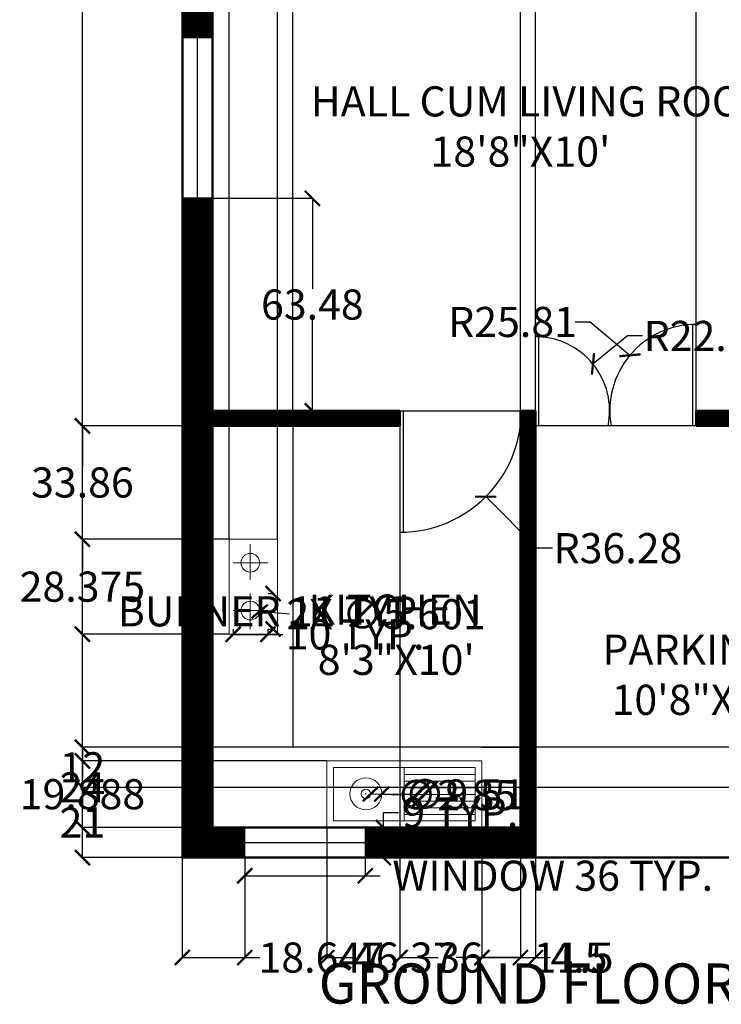
# Model space of a CAD drawing. Units: inches. Extents: x 104 to 466, y -74 to 547.
# Tile 1 of 4: x 110 to 320, y -74 to 220. Entities that reach past the tile are written whole.
import ezdxf

# ---------------------------------------------------------------- set-up
doc = ezdxf.new("R2010")
doc.units = ezdxf.units.IN
doc.header["$MEASUREMENT"] = 0
for name, color, linetype, lineweight in [('A-ANNO-DIMS', 2, 'Continuous', 18), ('A-ANNO-TEXT', 7, 'Continuous', 35), ('A-AREA-IDEN', 7, 'Continuous', 25), ('A-DOOR', 3, 'Continuous', 25), ('A-EQPM', 9, 'Continuous', 18), ('A-FLOR-CASE', 8, 'Continuous', 25), ('A-FLOR-FIXT', 8, 'Continuous', 18), ('A-GLAZ', 4, 'Continuous', 25), ('A-WALL', 7, 'Continuous', 50), ('A-WALL-PATT', 8, 'Continuous', 13)]:
    doc.layers.add(name, color=color, linetype=linetype, lineweight=lineweight)
doc.styles.get("Standard").update_dxf_attribs({"font": 'arial.ttf'})
doc.dimstyles.get("Standard").update_dxf_attribs({"dimtxt": 9, "dimasz": 4.5, "dimexe": 0.18, "dimexo": 0.0625, "dimgap": 0.09, "dimtad": 0, "dimtih": 1, "dimtoh": 1, "dimdec": 1, "dimzin": 0, "dimdsep": 46, "dimlunit": 4, "dimtxsty": 'Standard', "dimblk": 'ARCHTICK', "dimcen": 0.09, "dimadec": 0, "dimazin": 0, "dimtfac": 1, "dimtdec": 1, "dimtofl": 0, "dimtmove": 0, "dimatfit": 3, "dimfxl": 1, "dimtolj": 1, "dimtzin": 0, "dimarcsym": 0})

# ---------------------------------------------------------------- blocks, each defined once
blk = doc.blocks.new('WINDOW-48IN')
for p, q in [((0, 48), (9, 48)), ((0, 0), (0, 48)), ((4.5, 48), (4.5, 0)), ((9, 48), (9, 0)), ((9, 0), (0, 0))]:
    blk.add_line(p, q)
blk = doc.blocks.new('WINDOW-36IN')
for p, q in [((0, 9), (36, 9)), ((0, 0), (0, 9)), ((36, 9), (36, 0)), ((0, 4.5), (36, 4.5)), ((36, 0), (0, 0))]:
    blk.add_line(p, q)
blk = doc.blocks.new('COOKTOP-BURNER')
for q in [(5.16, 10.61), (0, 5.52), (5.16, 0), (10.39, 5.52)]:
    blk.add_line((5.16, 5.52), q)
blk.add_circle((5.16, 5.52), 2.8)
blk = doc.blocks.new('_ArchTick')
at = {"color": 0, "linetype": 'ByBlock', "const_width": 0.15}
blk.add_lwpolyline([(-0.5, -0.5), (0.5, 0.5)], dxfattribs=at)
blk = doc.blocks.new('*D9')
at = {"layer": 'A-ANNO-DIMS', "color": 0, "lineweight": -2, "transparency": 16777216}
for p, q in [((177.73, -30.52), (177.73, -36.04)), ((213.73, -30.52), (213.73, -36.04)), ((177.73, -35.86), (213.73, -35.86)), ((213.73, -35.86), (218.23, -35.86))]:
    blk.add_line(p, q, dxfattribs=at)
at = {"layer": 'Defpoints', "color": 0, "transparency": 16777216}
for p in [(177.73, -30.46), (213.73, -30.46), (213.73, -35.86)]:
    blk.add_point(p, dxfattribs=at)
at = {"layer": 'A-ANNO-DIMS', "color": 0, "lineweight": -2, "transparency": 16777216, "xscale": 4.5, "yscale": 4.5, "zscale": 4.5, "rotation": 180}
blk.add_blockref('_ArchTick', (177.73, -35.86), dxfattribs=at)
at = {"layer": 'A-ANNO-DIMS', "color": 0, "lineweight": -2, "transparency": 16777216, "xscale": 4.5, "yscale": 4.5, "zscale": 4.5}
blk.add_blockref('_ArchTick', (213.73, -35.86), dxfattribs=at)
at = {"layer": 'A-ANNO-DIMS', "color": 0, "transparency": 16777216, "insert": (269.74, -35.86), "char_height": 9, "attachment_point": 5}
blk.add_mtext('\\A1;WINDOW 36 TYP.', dxfattribs=at)
blk = doc.blocks.new('*D10')
at = {"layer": 'A-ANNO-DIMS', "color": 0, "lineweight": -2, "transparency": 16777216}
for p, q in [((219.13, -21.46), (219.13, -16.96)), ((219.13, -16.96), (223.63, -16.96)), ((213.79, -21.46), (219.31, -21.46)), ((219.13, -30.46), (219.13, -21.46)), ((213.79, -30.46), (219.31, -30.46))]:
    blk.add_line(p, q, dxfattribs=at)
at = {"layer": 'Defpoints', "color": 0, "transparency": 16777216}
for p in [(213.73, -21.46), (219.13, -21.46), (213.73, -30.46)]:
    blk.add_point(p, dxfattribs=at)
at = {"layer": 'A-ANNO-DIMS', "color": 0, "lineweight": -2, "transparency": 16777216, "xscale": 4.5, "yscale": 4.5, "zscale": 4.5}
for p, rotation in [((219.13, -21.46), 90), ((219.13, -30.46), 270)]:
    blk.add_blockref('_ArchTick', p, dxfattribs=dict(at, rotation=rotation))
at = {"layer": 'A-ANNO-DIMS', "color": 0, "transparency": 16777216, "insert": (242.13, -16.96), "char_height": 9, "attachment_point": 5}
blk.add_mtext('\\A1;9 TYP.', dxfattribs=at)
blk = doc.blocks.new('*D15')
at = {"layer": 'A-ANNO-DIMS', "color": 0, "lineweight": -2, "transparency": 16777216}
for p, q in [((184.68, 48.44), (186.39, 48.44)), ((186.21, 48.44), (186.21, 47.82)), ((186.21, 37.84), (186.21, 38.45)), ((184.68, 37.84), (186.39, 37.84))]:
    blk.add_line(p, q, dxfattribs=at)
at = {"layer": 'Defpoints', "color": 0, "transparency": 16777216}
for p in [(184.62, 48.44), (186.21, 48.44), (184.62, 37.84)]:
    blk.add_point(p, dxfattribs=at)
at = {"layer": 'A-ANNO-DIMS', "color": 0, "lineweight": -2, "transparency": 16777216, "xscale": 4.5, "yscale": 4.5, "zscale": 4.5}
for p, rotation in [((186.21, 48.44), 90), ((186.21, 37.84), 270)]:
    blk.add_blockref('_ArchTick', p, dxfattribs=dict(at, rotation=rotation))
at = {"layer": 'A-ANNO-DIMS', "color": 0, "transparency": 16777216, "insert": (186.21, 43.14), "char_height": 9, "attachment_point": 5}
blk.add_mtext('\\A1;BURNER 11 TYP.', dxfattribs=at)
blk = doc.blocks.new('*D16')
at = {"layer": 'A-ANNO-DIMS', "color": 0, "lineweight": -2, "transparency": 16777216}
for p, q in [((174.23, 37.77), (174.23, 36.06)), ((174.23, 36.24), (184.62, 36.24)), ((184.62, 37.77), (184.62, 36.06)), ((184.62, 36.24), (189.12, 36.24))]:
    blk.add_line(p, q, dxfattribs=at)
at = {"layer": 'Defpoints', "color": 0, "transparency": 16777216}
for p in [(174.23, 37.84), (184.62, 37.84), (184.62, 36.24)]:
    blk.add_point(p, dxfattribs=at)
at = {"layer": 'A-ANNO-DIMS', "color": 0, "lineweight": -2, "transparency": 16777216, "xscale": 4.5, "yscale": 4.5, "zscale": 4.5, "rotation": 180}
blk.add_blockref('_ArchTick', (174.23, 36.24), dxfattribs=at)
at = {"layer": 'A-ANNO-DIMS', "color": 0, "lineweight": -2, "transparency": 16777216, "xscale": 4.5, "yscale": 4.5, "zscale": 4.5}
blk.add_blockref('_ArchTick', (184.62, 36.24), dxfattribs=at)
at = {"layer": 'A-ANNO-DIMS', "color": 0, "transparency": 16777216, "insert": (210.69, 36.24), "char_height": 9, "attachment_point": 5}
blk.add_mtext('\\A1;10 TYP.', dxfattribs=at)
blk = doc.blocks.new('*D18')
at = {"layer": 'A-ANNO-DIMS', "color": 0, "lineweight": -2, "transparency": 16777216}
for p, q in [((159.02, 511.04), (129.05, 511.04)), ((129.23, 511.04), (129.23, 244.98)), ((129.23, -30.46), (129.23, 235.61)), ((159.02, -30.46), (129.05, -30.46))]:
    blk.add_line(p, q, dxfattribs=at)
at = {"layer": 'Defpoints', "color": 0, "transparency": 16777216}
for p in [(129.23, 511.04), (159.08, 511.04), (159.08, -30.46)]:
    blk.add_point(p, dxfattribs=at)
at = {"layer": 'A-ANNO-DIMS', "color": 0, "lineweight": -2, "transparency": 16777216, "xscale": 4.5, "yscale": 4.5, "zscale": 4.5}
for p, rotation in [((129.23, 511.04), 90), ((129.23, -30.46), 270)]:
    blk.add_blockref('_ArchTick', p, dxfattribs=dict(at, rotation=rotation))
at = {"layer": 'A-ANNO-DIMS', "color": 0, "transparency": 16777216, "insert": (129.23, 240.29), "char_height": 9, "attachment_point": 5}
blk.add_mtext('\\A1;541.5', dxfattribs=at)
blk = doc.blocks.new('*D19')
at = {"layer": 'A-ANNO-DIMS', "color": 0, "lineweight": -2, "transparency": 16777216}
for p, q in [((159.08, -30.52), (159.08, -60.49)), ((177.73, -30.52), (177.73, -60.49)), ((159.08, -60.31), (177.73, -60.31)), ((177.73, -60.31), (182.23, -60.31))]:
    blk.add_line(p, q, dxfattribs=at)
at = {"layer": 'Defpoints', "color": 0, "transparency": 16777216}
for p in [(159.08, -30.46), (177.73, -30.46), (177.73, -60.31)]:
    blk.add_point(p, dxfattribs=at)
at = {"layer": 'A-ANNO-DIMS', "color": 0, "lineweight": -2, "transparency": 16777216, "xscale": 4.5, "yscale": 4.5, "zscale": 4.5, "rotation": 180}
blk.add_blockref('_ArchTick', (159.08, -60.31), dxfattribs=at)
at = {"layer": 'A-ANNO-DIMS', "color": 0, "lineweight": -2, "transparency": 16777216, "xscale": 4.5, "yscale": 4.5, "zscale": 4.5}
blk.add_blockref('_ArchTick', (177.73, -60.31), dxfattribs=at)
at = {"layer": 'A-ANNO-DIMS', "color": 0, "transparency": 16777216, "insert": (200.58, -60.31), "char_height": 9, "attachment_point": 5}
blk.add_mtext('\\A1;18.647', dxfattribs=at)
blk = doc.blocks.new('*D21')
at = {"layer": 'A-ANNO-DIMS', "color": 0, "lineweight": -2, "transparency": 16777216}
for p, q in [((168.15, 166.52), (198.11, 166.52)), ((197.93, 166.52), (197.93, 139.47)), ((197.93, 103.04), (197.93, 130.1)), ((168.15, 103.04), (198.11, 103.04))]:
    blk.add_line(p, q, dxfattribs=at)
at = {"layer": 'Defpoints', "color": 0, "transparency": 16777216}
for p in [(168.08, 166.52), (168.08, 103.04), (197.93, 103.04)]:
    blk.add_point(p, dxfattribs=at)
at = {"layer": 'A-ANNO-DIMS', "color": 0, "lineweight": -2, "transparency": 16777216, "xscale": 4.5, "yscale": 4.5, "zscale": 4.5}
for p, rotation in [((197.93, 166.52), 90), ((197.93, 103.04), 270)]:
    blk.add_blockref('_ArchTick', p, dxfattribs=dict(at, rotation=rotation))
at = {"layer": 'A-ANNO-DIMS', "color": 0, "transparency": 16777216, "insert": (197.93, 134.78), "char_height": 9, "attachment_point": 5}
blk.add_mtext('\\A1;63.48', dxfattribs=at)
blk = doc.blocks.new('*D26')
at = {"layer": 'A-ANNO-DIMS', "color": 0, "lineweight": -2, "transparency": 16777216}
for p, q in [((168.08, 98.61), (168.08, 541.07)), ((168.08, 540.89), (207.59, 540.89)), ((260.08, 540.89), (220.57, 540.89)), ((260.08, 103.11), (260.08, 541.07))]:
    blk.add_line(p, q, dxfattribs=at)
at = {"layer": 'Defpoints', "color": 0, "transparency": 16777216}
for p in [(260.08, 540.89), (260.08, 103.04), (168.08, 98.54)]:
    blk.add_point(p, dxfattribs=at)
at = {"layer": 'A-ANNO-DIMS', "color": 0, "lineweight": -2, "transparency": 16777216, "xscale": 4.5, "yscale": 4.5, "zscale": 4.5, "rotation": 180}
blk.add_blockref('_ArchTick', (168.08, 540.89), dxfattribs=at)
at = {"layer": 'A-ANNO-DIMS', "color": 0, "lineweight": -2, "transparency": 16777216, "xscale": 4.5, "yscale": 4.5, "zscale": 4.5}
blk.add_blockref('_ArchTick', (260.08, 540.89), dxfattribs=at)
at = {"layer": 'A-ANNO-DIMS', "color": 0, "transparency": 16777216, "insert": (214.08, 540.89), "char_height": 9, "attachment_point": 5}
blk.add_mtext('\\A1;92', dxfattribs=at)
blk = doc.blocks.new('*D27')
at = {"layer": 'A-ANNO-DIMS', "color": 0, "lineweight": -2, "transparency": 16777216}
for p, q in [((260.08, -21.52), (260.08, -60.49)), ((264.58, -30.52), (264.58, -60.49)), ((260.08, -60.31), (264.58, -60.31)), ((264.58, -60.31), (269.08, -60.31))]:
    blk.add_line(p, q, dxfattribs=at)
at = {"layer": 'Defpoints', "color": 0, "transparency": 16777216}
for p in [(260.08, -21.46), (264.58, -30.46), (264.58, -60.31)]:
    blk.add_point(p, dxfattribs=at)
at = {"layer": 'A-ANNO-DIMS', "color": 0, "lineweight": -2, "transparency": 16777216, "xscale": 4.5, "yscale": 4.5, "zscale": 4.5, "rotation": 180}
blk.add_blockref('_ArchTick', (260.08, -60.31), dxfattribs=at)
at = {"layer": 'A-ANNO-DIMS', "color": 0, "lineweight": -2, "transparency": 16777216, "xscale": 4.5, "yscale": 4.5, "zscale": 4.5}
blk.add_blockref('_ArchTick', (264.58, -60.31), dxfattribs=at)
at = {"layer": 'A-ANNO-DIMS', "color": 0, "transparency": 16777216, "insert": (277.58, -60.31), "char_height": 9, "attachment_point": 5}
blk.add_mtext('\\A1;4.5', dxfattribs=at)
blk = doc.blocks.new('*D30')
at = {"layer": 'A-ANNO-DIMS', "color": 0, "lineweight": -2, "transparency": 16777216}
for p, q in [((368.52, 2.54), (129.05, 2.54)), ((129.23, 2.54), (129.23, 1.15)), ((129.23, -9.46), (129.23, -8.06)), ((368.52, -9.46), (129.05, -9.46))]:
    blk.add_line(p, q, dxfattribs=at)
at = {"layer": 'Defpoints', "color": 0, "transparency": 16777216}
for p in [(129.23, 2.54), (368.58, 2.54), (368.58, -9.46)]:
    blk.add_point(p, dxfattribs=at)
at = {"layer": 'A-ANNO-DIMS', "color": 0, "lineweight": -2, "transparency": 16777216, "xscale": 4.5, "yscale": 4.5, "zscale": 4.5}
for p, rotation in [((129.23, 2.54), 90), ((129.23, -9.46), 270)]:
    blk.add_blockref('_ArchTick', p, dxfattribs=dict(at, rotation=rotation))
at = {"layer": 'A-ANNO-DIMS', "color": 0, "transparency": 16777216, "insert": (129.23, -3.46), "char_height": 9, "attachment_point": 5}
blk.add_mtext('\\A1;12', dxfattribs=at)
blk = doc.blocks.new('*D31')
at = {"layer": 'A-ANNO-DIMS', "color": 0, "lineweight": -2, "transparency": 16777216}
for p, q in [((168.08, 98.61), (168.08, 541.07)), ((168.08, 540.89), (173.49, 540.89)), ((192.08, 540.89), (186.68, 540.89)), ((192.08, 98.61), (192.08, 541.07))]:
    blk.add_line(p, q, dxfattribs=at)
at = {"layer": 'Defpoints', "color": 0, "transparency": 16777216}
for p in [(192.08, 540.89), (168.08, 98.54), (192.08, 98.54)]:
    blk.add_point(p, dxfattribs=at)
at = {"layer": 'A-ANNO-DIMS', "color": 0, "lineweight": -2, "transparency": 16777216, "xscale": 4.5, "yscale": 4.5, "zscale": 4.5, "rotation": 180}
blk.add_blockref('_ArchTick', (168.08, 540.89), dxfattribs=at)
at = {"layer": 'A-ANNO-DIMS', "color": 0, "lineweight": -2, "transparency": 16777216, "xscale": 4.5, "yscale": 4.5, "zscale": 4.5}
blk.add_blockref('_ArchTick', (192.08, 540.89), dxfattribs=at)
at = {"layer": 'A-ANNO-DIMS', "color": 0, "transparency": 16777216, "insert": (180.08, 540.89), "char_height": 9, "attachment_point": 5}
blk.add_mtext('\\A1;24', dxfattribs=at)
blk = doc.blocks.new('*D32')
at = {"layer": 'A-ANNO-DIMS', "color": 0, "lineweight": -2, "transparency": 16777216}
for p, q in [((260.02, 2.54), (129.05, 2.54)), ((129.23, 2.54), (129.23, -4.85)), ((129.23, -21.46), (129.23, -14.06)), ((260.02, -21.46), (129.05, -21.46))]:
    blk.add_line(p, q, dxfattribs=at)
at = {"layer": 'Defpoints', "color": 0, "transparency": 16777216}
for p in [(129.23, 2.54), (260.08, 2.54), (260.08, -21.46)]:
    blk.add_point(p, dxfattribs=at)
at = {"layer": 'A-ANNO-DIMS', "color": 0, "lineweight": -2, "transparency": 16777216, "xscale": 4.5, "yscale": 4.5, "zscale": 4.5}
for p, rotation in [((129.23, 2.54), 90), ((129.23, -21.46), 270)]:
    blk.add_blockref('_ArchTick', p, dxfattribs=dict(at, rotation=rotation))
at = {"layer": 'A-ANNO-DIMS', "color": 0, "transparency": 16777216, "insert": (129.23, -9.46), "char_height": 9, "attachment_point": 5}
blk.add_mtext('\\A1;24', dxfattribs=at)
blk = doc.blocks.new('*D33')
at = {"layer": 'A-ANNO-DIMS', "color": 0, "lineweight": -2, "transparency": 16777216}
for p, q in [((202.22, -21.52), (202.22, -60.49)), ((248.58, -21.52), (248.58, -60.49)), ((202.22, -60.31), (209.94, -60.31)), ((248.58, -60.31), (240.86, -60.31))]:
    blk.add_line(p, q, dxfattribs=at)
at = {"layer": 'Defpoints', "color": 0, "transparency": 16777216}
for p in [(202.22, -21.46), (248.58, -21.46), (248.58, -60.31)]:
    blk.add_point(p, dxfattribs=at)
at = {"layer": 'A-ANNO-DIMS', "color": 0, "lineweight": -2, "transparency": 16777216, "xscale": 4.5, "yscale": 4.5, "zscale": 4.5, "rotation": 180}
blk.add_blockref('_ArchTick', (202.22, -60.31), dxfattribs=at)
at = {"layer": 'A-ANNO-DIMS', "color": 0, "lineweight": -2, "transparency": 16777216, "xscale": 4.5, "yscale": 4.5, "zscale": 4.5}
blk.add_blockref('_ArchTick', (248.58, -60.31), dxfattribs=at)
at = {"layer": 'A-ANNO-DIMS', "color": 0, "transparency": 16777216, "insert": (225.4, -60.31), "char_height": 9, "attachment_point": 5}
blk.add_mtext('\\A1;46.37', dxfattribs=at)
blk = doc.blocks.new('*D34')
at = {"layer": 'A-ANNO-DIMS', "color": 0, "lineweight": -2, "transparency": 16777216}
for p, q in [((248.58, -21.52), (248.58, -60.49)), ((260.08, -21.52), (260.08, -60.49)), ((248.58, -60.31), (260.08, -60.31)), ((260.08, -60.31), (264.58, -60.31))]:
    blk.add_line(p, q, dxfattribs=at)
at = {"layer": 'Defpoints', "color": 0, "transparency": 16777216}
for p in [(248.58, -21.46), (260.08, -21.46), (260.08, -60.31)]:
    blk.add_point(p, dxfattribs=at)
at = {"layer": 'A-ANNO-DIMS', "color": 0, "lineweight": -2, "transparency": 16777216, "xscale": 4.5, "yscale": 4.5, "zscale": 4.5, "rotation": 180}
blk.add_blockref('_ArchTick', (248.58, -60.31), dxfattribs=at)
at = {"layer": 'A-ANNO-DIMS', "color": 0, "lineweight": -2, "transparency": 16777216, "xscale": 4.5, "yscale": 4.5, "zscale": 4.5}
blk.add_blockref('_ArchTick', (260.08, -60.31), dxfattribs=at)
at = {"layer": 'A-ANNO-DIMS', "color": 0, "transparency": 16777216, "insert": (275.97, -60.31), "char_height": 9, "attachment_point": 5}
blk.add_mtext('\\A1;11.5', dxfattribs=at)
blk = doc.blocks.new('*D35')
at = {"layer": 'A-ANNO-DIMS', "color": 0, "lineweight": -2, "transparency": 16777216}
for p, q in [((202.16, -1.57), (129.05, -1.57)), ((129.23, -1.57), (129.23, -6.83)), ((129.23, -21.46), (129.23, -16.2)), ((202.16, -21.46), (129.05, -21.46))]:
    blk.add_line(p, q, dxfattribs=at)
at = {"layer": 'Defpoints', "color": 0, "transparency": 16777216}
for p in [(129.23, -1.57), (202.22, -1.57), (202.22, -21.46)]:
    blk.add_point(p, dxfattribs=at)
at = {"layer": 'A-ANNO-DIMS', "color": 0, "lineweight": -2, "transparency": 16777216, "xscale": 4.5, "yscale": 4.5, "zscale": 4.5}
for p, rotation in [((129.23, -1.57), 90), ((129.23, -21.46), 270)]:
    blk.add_blockref('_ArchTick', p, dxfattribs=dict(at, rotation=rotation))
at = {"layer": 'A-ANNO-DIMS', "color": 0, "transparency": 16777216, "insert": (129.23, -11.51), "char_height": 9, "attachment_point": 5}
blk.add_mtext('\\A1;19.888', dxfattribs=at)
blk = doc.blocks.new('*D36')
at = {"layer": 'A-ANNO-DIMS', "color": 0, "lineweight": -2, "transparency": 16777216}
for p, q in [((392.52, -9.46), (129.05, -9.46)), ((129.23, -9.46), (129.23, -15.35)), ((129.23, -30.46), (129.23, -24.56)), ((392.52, -30.46), (129.05, -30.46))]:
    blk.add_line(p, q, dxfattribs=at)
at = {"layer": 'Defpoints', "color": 0, "transparency": 16777216}
for p in [(392.58, -9.46), (129.23, -30.46), (392.58, -30.46)]:
    blk.add_point(p, dxfattribs=at)
at = {"layer": 'A-ANNO-DIMS', "color": 0, "lineweight": -2, "transparency": 16777216, "xscale": 4.5, "yscale": 4.5, "zscale": 4.5}
for p, rotation in [((129.23, -9.46), 90), ((129.23, -30.46), 270)]:
    blk.add_blockref('_ArchTick', p, dxfattribs=dict(at, rotation=rotation))
at = {"layer": 'A-ANNO-DIMS', "color": 0, "transparency": 16777216, "insert": (129.23, -19.96), "char_height": 9, "attachment_point": 5}
blk.add_mtext('\\A1;21', dxfattribs=at)
blk = doc.blocks.new('*D37')
at = {"layer": 'A-ANNO-DIMS', "color": 0, "lineweight": -2, "transparency": 16777216}
for p, q in [((264.58, 98.61), (264.58, 541.07)), ((264.58, 540.89), (281.86, 540.89)), ((312.58, 540.89), (295.31, 540.89)), ((312.58, 98.61), (312.58, 541.07))]:
    blk.add_line(p, q, dxfattribs=at)
at = {"layer": 'Defpoints', "color": 0, "transparency": 16777216}
for p in [(312.58, 540.89), (264.58, 98.54), (312.58, 98.54)]:
    blk.add_point(p, dxfattribs=at)
at = {"layer": 'A-ANNO-DIMS', "color": 0, "lineweight": -2, "transparency": 16777216, "xscale": 4.5, "yscale": 4.5, "zscale": 4.5, "rotation": 180}
blk.add_blockref('_ArchTick', (264.58, 540.89), dxfattribs=at)
at = {"layer": 'A-ANNO-DIMS', "color": 0, "lineweight": -2, "transparency": 16777216, "xscale": 4.5, "yscale": 4.5, "zscale": 4.5}
blk.add_blockref('_ArchTick', (312.58, 540.89), dxfattribs=at)
at = {"layer": 'A-ANNO-DIMS', "color": 0, "transparency": 16777216, "insert": (288.58, 540.89), "char_height": 9, "attachment_point": 5}
blk.add_mtext('\\A1;48', dxfattribs=at)
blk = doc.blocks.new('*D38')
at = {"layer": 'A-ANNO-DIMS', "color": 0, "lineweight": -2, "transparency": 16777216}
for p, q in [((224.08, 98.48), (224.08, -60.49)), ((260.08, 98.48), (260.08, -60.49)), ((224.08, -60.31), (235.55, -60.31)), ((260.08, -60.31), (248.61, -60.31))]:
    blk.add_line(p, q, dxfattribs=at)
at = {"layer": 'Defpoints', "color": 0, "transparency": 16777216}
for p in [(224.08, 98.54), (260.08, 98.54), (260.08, -60.31)]:
    blk.add_point(p, dxfattribs=at)
at = {"layer": 'A-ANNO-DIMS', "color": 0, "lineweight": -2, "transparency": 16777216, "xscale": 4.5, "yscale": 4.5, "zscale": 4.5, "rotation": 180}
blk.add_blockref('_ArchTick', (224.08, -60.31), dxfattribs=at)
at = {"layer": 'A-ANNO-DIMS', "color": 0, "lineweight": -2, "transparency": 16777216, "xscale": 4.5, "yscale": 4.5, "zscale": 4.5}
blk.add_blockref('_ArchTick', (260.08, -60.31), dxfattribs=at)
at = {"layer": 'A-ANNO-DIMS', "color": 0, "transparency": 16777216, "insert": (242.08, -60.31), "char_height": 9, "attachment_point": 5}
blk.add_mtext('\\A1;36', dxfattribs=at)
blk = doc.blocks.new('*D50')
at = {"layer": 'A-ANNO-DIMS', "color": 0, "lineweight": -2, "transparency": 16777216}
for p, q in [((173.04, 64.75), (173.04, 541.07)), ((173.04, 540.89), (187.51, 540.89)), ((187.51, 64.75), (187.51, 541.07)), ((187.51, 540.89), (192.01, 540.89))]:
    blk.add_line(p, q, dxfattribs=at)
at = {"layer": 'Defpoints', "color": 0, "transparency": 16777216}
for p in [(187.51, 540.89), (173.04, 64.69), (187.51, 64.69)]:
    blk.add_point(p, dxfattribs=at)
at = {"layer": 'A-ANNO-DIMS', "color": 0, "lineweight": -2, "transparency": 16777216, "xscale": 4.5, "yscale": 4.5, "zscale": 4.5, "rotation": 180}
blk.add_blockref('_ArchTick', (173.04, 540.89), dxfattribs=at)
at = {"layer": 'A-ANNO-DIMS', "color": 0, "lineweight": -2, "transparency": 16777216, "xscale": 4.5, "yscale": 4.5, "zscale": 4.5}
blk.add_blockref('_ArchTick', (187.51, 540.89), dxfattribs=at)
at = {"layer": 'A-ANNO-DIMS', "color": 0, "transparency": 16777216, "insert": (210.36, 540.89), "char_height": 9, "attachment_point": 5}
blk.add_mtext('\\A1;14.476', dxfattribs=at)
blk = doc.blocks.new('*D51')
at = {"layer": 'A-ANNO-DIMS', "color": 0, "lineweight": -2, "transparency": 16777216}
for p, q in [((172.97, 64.69), (129.05, 64.69)), ((129.23, 64.69), (129.23, 55.19)), ((129.23, 36.31), (129.23, 45.81)), ((172.97, 36.31), (129.05, 36.31))]:
    blk.add_line(p, q, dxfattribs=at)
at = {"layer": 'Defpoints', "color": 0, "transparency": 16777216}
for p in [(129.23, 64.69), (173.04, 64.69), (173.04, 36.31)]:
    blk.add_point(p, dxfattribs=at)
at = {"layer": 'A-ANNO-DIMS', "color": 0, "lineweight": -2, "transparency": 16777216, "xscale": 4.5, "yscale": 4.5, "zscale": 4.5}
for p, rotation in [((129.23, 64.69), 90), ((129.23, 36.31), 270)]:
    blk.add_blockref('_ArchTick', p, dxfattribs=dict(at, rotation=rotation))
at = {"layer": 'A-ANNO-DIMS', "color": 0, "transparency": 16777216, "insert": (129.23, 50.5), "char_height": 9, "attachment_point": 5}
blk.add_mtext('\\A1;28.375', dxfattribs=at)
blk = doc.blocks.new('*D52')
at = {"layer": 'A-ANNO-DIMS', "color": 0, "lineweight": -2, "transparency": 16777216}
for p, q in [((168.02, 98.54), (129.05, 98.54)), ((129.23, 98.54), (129.23, 86.3)), ((129.23, 64.69), (129.23, 76.93)), ((172.97, 64.69), (129.05, 64.69))]:
    blk.add_line(p, q, dxfattribs=at)
at = {"layer": 'Defpoints', "color": 0, "transparency": 16777216}
for p in [(129.23, 98.54), (168.08, 98.54), (173.04, 64.69)]:
    blk.add_point(p, dxfattribs=at)
at = {"layer": 'A-ANNO-DIMS', "color": 0, "lineweight": -2, "transparency": 16777216, "xscale": 4.5, "yscale": 4.5, "zscale": 4.5}
for p, rotation in [((129.23, 98.54), 90), ((129.23, 64.69), 270)]:
    blk.add_blockref('_ArchTick', p, dxfattribs=dict(at, rotation=rotation))
at = {"layer": 'A-ANNO-DIMS', "color": 0, "transparency": 16777216, "insert": (129.23, 81.62), "char_height": 9, "attachment_point": 5}
blk.add_mtext('\\A1;33.86', dxfattribs=at)
blk = doc.blocks.new('*D53')
at = {"layer": 'A-ANNO-DIMS', "color": 0, "lineweight": -2, "transparency": 16777216}
for p, q in [((168.08, 98.61), (168.08, 541.07)), ((168.08, 540.89), (173.04, 540.89)), ((173.04, 64.75), (173.04, 541.07)), ((173.04, 540.89), (177.54, 540.89))]:
    blk.add_line(p, q, dxfattribs=at)
at = {"layer": 'Defpoints', "color": 0, "transparency": 16777216}
for p in [(173.04, 540.89), (168.08, 98.54), (173.04, 64.69)]:
    blk.add_point(p, dxfattribs=at)
at = {"layer": 'A-ANNO-DIMS', "color": 0, "lineweight": -2, "transparency": 16777216, "xscale": 4.5, "yscale": 4.5, "zscale": 4.5, "rotation": 180}
blk.add_blockref('_ArchTick', (168.08, 540.89), dxfattribs=at)
at = {"layer": 'A-ANNO-DIMS', "color": 0, "lineweight": -2, "transparency": 16777216, "xscale": 4.5, "yscale": 4.5, "zscale": 4.5}
blk.add_blockref('_ArchTick', (173.04, 540.89), dxfattribs=at)
at = {"layer": 'A-ANNO-DIMS', "color": 0, "transparency": 16777216, "insert": (192.99, 540.89), "char_height": 9, "attachment_point": 5}
blk.add_mtext('\\A1;4.953', dxfattribs=at)
blk = doc.blocks.new('*D58')
at = {"layer": 'A-ANNO-DIMS', "color": 0, "lineweight": -2, "transparency": 16777216}
for p, q in [((213.82, -11.4), (214, -11.4)), ((213.91, -11.49), (213.91, -11.31)), ((227.67, -11.55), (218.67, -11.45))]:
    blk.add_line(p, q, dxfattribs=at)
at = {"layer": 'Defpoints', "color": 0, "transparency": 16777216}
for p in [(209.16, -11.35), (218.67, -11.45)]:
    blk.add_point(p, dxfattribs=at)
at = {"layer": 'A-ANNO-DIMS', "color": 0, "lineweight": -2, "transparency": 16777216, "xscale": 4.5, "yscale": 4.5, "zscale": 4.5, "rotation": 179.3781113712907}
blk.add_blockref('_ArchTick', (218.67, -11.45), dxfattribs=at)
at = {"layer": 'A-ANNO-DIMS', "color": 0, "transparency": 16777216, "insert": (243.47, -11.55), "char_height": 9, "attachment_point": 5}
blk.add_mtext('\\A1;∅9.51', dxfattribs=at)
blk = doc.blocks.new('*D59')
at = {"layer": 'A-ANNO-DIMS', "color": 0, "lineweight": -2, "transparency": 16777216}
for p, q in [((213.82, -11.4), (214, -11.4)), ((213.91, -11.49), (213.91, -11.31)), ((224.33, -11.78), (215.34, -11.45))]:
    blk.add_line(p, q, dxfattribs=at)
at = {"layer": 'Defpoints', "color": 0, "transparency": 16777216}
for p in [(212.49, -11.35), (215.34, -11.45)]:
    blk.add_point(p, dxfattribs=at)
at = {"layer": 'A-ANNO-DIMS', "color": 0, "lineweight": -2, "transparency": 16777216, "xscale": 4.5, "yscale": 4.5, "zscale": 4.5, "rotation": 177.9170163063177}
blk.add_blockref('_ArchTick', (215.34, -11.45), dxfattribs=at)
at = {"layer": 'A-ANNO-DIMS', "color": 0, "transparency": 16777216, "insert": (241.04, -11.78), "char_height": 9, "attachment_point": 5}
blk.add_mtext('\\A1;∅2.85', dxfattribs=at)
blk = doc.blocks.new('*D60')
at = {"layer": 'A-ANNO-DIMS', "color": 0, "lineweight": -2, "transparency": 16777216}
for p, q in [((179.3, 43.36), (179.48, 43.36)), ((179.39, 43.27), (179.39, 43.45)), ((191.14, 42.27), (182.18, 43.1))]:
    blk.add_line(p, q, dxfattribs=at)
at = {"layer": 'Defpoints', "color": 0, "transparency": 16777216}
for p in [(176.6, 43.62), (182.18, 43.1)]:
    blk.add_point(p, dxfattribs=at)
at = {"layer": 'A-ANNO-DIMS', "color": 0, "lineweight": -2, "transparency": 16777216, "xscale": 4.5, "yscale": 4.5, "zscale": 4.5, "rotation": 174.7039830258441}
blk.add_blockref('_ArchTick', (182.18, 43.1), dxfattribs=at)
at = {"layer": 'A-ANNO-DIMS', "color": 0, "transparency": 16777216, "insert": (219.95, 42.27), "char_height": 9, "attachment_point": 5}
blk.add_mtext('\\A1;2X ∅5.601', dxfattribs=at)
blk = doc.blocks.new('*D63')
at = {"layer": 'A-ANNO-DIMS', "color": 0, "lineweight": -2, "transparency": 16777216}
for p, q in [((223.99, 103.04), (224.17, 103.04)), ((224.08, 102.95), (224.08, 103.13)), ((265.13, 62), (249.74, 77.39)), ((269.63, 62), (265.13, 62))]:
    blk.add_line(p, q, dxfattribs=at)
at = {"layer": 'Defpoints', "color": 0, "transparency": 16777216}
for p in [(224.08, 103.04), (249.74, 77.39)]:
    blk.add_point(p, dxfattribs=at)
at = {"layer": 'A-ANNO-DIMS', "color": 0, "lineweight": -2, "transparency": 16777216, "xscale": 4.5, "yscale": 4.5, "zscale": 4.5, "rotation": 134.9998280274367}
blk.add_blockref('_ArchTick', (249.74, 77.39), dxfattribs=at)
at = {"layer": 'A-ANNO-DIMS', "color": 0, "transparency": 16777216, "insert": (289.22, 62), "char_height": 9, "attachment_point": 5}
blk.add_mtext('\\A1;R36.28', dxfattribs=at)
blk = doc.blocks.new('*D66')
at = {"layer": 'A-ANNO-DIMS', "color": 0, "lineweight": -2, "transparency": 16777216}
for p, q in [((276.44, 129.58), (280.94, 129.58)), ((280.94, 129.58), (292.81, 119.63)), ((312.49, 103.04), (312.67, 103.04)), ((312.58, 102.95), (312.58, 103.13))]:
    blk.add_line(p, q, dxfattribs=at)
at = {"layer": 'Defpoints', "color": 0, "transparency": 16777216}
for p in [(292.81, 119.63), (312.58, 103.04)]:
    blk.add_point(p, dxfattribs=at)
at = {"layer": 'A-ANNO-DIMS', "color": 0, "lineweight": -2, "transparency": 16777216, "xscale": 4.5, "yscale": 4.5, "zscale": 4.5, "rotation": 320.0206828302677}
blk.add_blockref('_ArchTick', (292.81, 119.63), dxfattribs=at)
at = {"layer": 'A-ANNO-DIMS', "color": 0, "transparency": 16777216, "insert": (257.73, 129.58), "char_height": 9, "attachment_point": 5}
blk.add_mtext('\\A1;R25.81', dxfattribs=at)
blk = doc.blocks.new('*D67')
at = {"layer": 'A-ANNO-DIMS', "color": 0, "lineweight": -2, "transparency": 16777216}
for p, q in [((292.06, 125.4), (281.76, 117.02)), ((296.56, 125.4), (292.06, 125.4)), ((264.49, 103.04), (264.67, 103.04)), ((264.58, 102.95), (264.58, 103.13))]:
    blk.add_line(p, q, dxfattribs=at)
at = {"layer": 'Defpoints', "color": 0, "transparency": 16777216}
for p in [(281.76, 117.02), (264.58, 103.04)]:
    blk.add_point(p, dxfattribs=at)
at = {"layer": 'A-ANNO-DIMS', "color": 0, "lineweight": -2, "transparency": 16777216, "xscale": 4.5, "yscale": 4.5, "zscale": 4.5, "rotation": 219.1362079065188}
blk.add_blockref('_ArchTick', (281.76, 117.02), dxfattribs=at)
at = {"layer": 'A-ANNO-DIMS', "color": 0, "transparency": 16777216, "insert": (316.12, 125.4), "char_height": 9, "attachment_point": 5}
blk.add_mtext('\\A1;R22.14', dxfattribs=at)

msp = doc.modelspace()

# ---------------------------------------------------------------- hatches: boundary and pattern name
at = {"layer": 'A-WALL-PATT'}
h = msp.add_hatch(dxfattribs=at)
h.set_pattern_fill('ANSI31', color=256)
h.set_pattern_definition([(45, (-366.28003, -301.99136), (-0.088388348, 0.088388348), [])])
h.paths.add_polyline_path([(401.5842, 137.0851), (401.5842, 171.2112), (392.5842, 171.2112), (392.5842, 167.545), (332.0842, 167.545), (332.0842, 137.0851), (332.0842, 103.045), (312.5842, 103.045), (312.5842, 98.545), (392.5842, 98.545), (392.5842, -9.455), (392.5842, -30.455), (401.5842, -30.455), (401.5842, 31.361)])
h.paths.add_polyline_path([(392.5842, 103.045), (336.5842, 103.045), (336.5842, 137.0851), (336.5842, 163.045), (392.5842, 163.045), (392.5842, 137.0851)], flags=16)
h.paths.add_polyline_path([(401.5842, 292.5416), (392.5842, 292.5416), (392.5842, 227.545), (248.5842, 227.545), (248.5842, 232.045), (244.0842, 232.045), (244.0842, 223.045), (248.5842, 223.045), (392.5842, 223.045), (392.5842, 219.2112), (401.5842, 219.2112)])
h.paths.add_polyline_path([(401.5842, 388.2533), (392.5842, 388.2533), (392.5842, 370.045), (340.5842, 370.045), (340.5842, 369.865, -0.03576944), (340.8936, 365.545), (392.5842, 365.545), (392.5842, 340.5416), (401.5842, 340.5416)], flags=17)
h.paths.add_polyline_path([(401.5842, 453.4958), (392.5842, 453.4958), (392.5842, 438.045), (310.5842, 438.045), (310.5842, 467.545), (306.0842, 467.545), (306.0842, 370.045), (208.837, 370.045, -0.03088397), (209.1152, 365.545), (244.0842, 365.545), (244.0842, 274.587, -0.0265002), (248.5842, 274.3483), (248.5842, 365.545), (306.0842, 365.545), (310.5842, 365.545), (310.5842, 370.045), (310.5842, 433.545), (392.5842, 433.545), (392.5842, 424.2533), (401.5842, 424.2533)])
h.paths.add_polyline_path([(168.0842, 365.545), (172.5842, 365.545), (172.5842, 370.045), (168.0842, 370.045), (168.0842, 414.671), (159.0842, 414.671), (159.0842, 214.5244), (168.0842, 214.5244)])
h.paths.add_polyline_path([(168.0842, 98.545), (224.0842, 98.545), (224.0842, 103.045), (168.0842, 103.045), (168.0842, 137.0851), (168.0842, 166.5244), (159.0842, 166.5244), (159.0842, 137.0851), (159.0842, 43.0309), (159.0842, -30.455), (168.0842, -30.455), (177.7316, -30.455), (177.7316, -21.455), (168.0842, -21.455), (168.0842, 35.9487)])
h.paths.add_polyline_path([(264.5842, -21.455), (264.5842, 98.545), (264.5842, 103.045), (260.3643, 103.045, -0.03109877), (260.0842, 98.545), (260.0842, -21.455), (248.5842, -21.455), (213.7316, -21.455), (213.7316, -30.455), (248.5842, -30.455), (264.5842, -30.455)])
h.paths.add_polyline_path([(401.5842, 511.045), (159.0842, 511.045), (159.0842, 462.671), (168.0842, 462.671), (168.0842, 502.045), (306.0842, 502.045), (306.0842, 497.545), (310.5842, 497.545), (310.5842, 502.045), (392.5842, 502.045), (392.5842, 489.4958), (401.5842, 489.4958)])

# ---------------------------------------------------------------- linework, layer by layer
at = {"layer": 'A-DOOR'}
for p, q in [((311.5842, 98.545), (311.5842, 128.8337)), ((312.5842, 98.545), (312.5842, 128.853)), ((264.5842, 98.545), (264.5842, 125.1851)), ((265.5842, 98.545), (265.5842, 125.1625)), ((224.0842, 103.045), (260.0842, 103.045)), ((224.0842, 103.045), (224.0842, 66.7648)), ((225.0842, 103.045), (225.0842, 66.7786)), ((312.5842, 98.545), (264.5842, 98.545))]:
    msp.add_line(p, q, dxfattribs=at)
for centre, radius, start, end in [((312.5842, 103.045), 25.808, 90, 190.041662), ((264.5842, 103.045), 22.1401, 348.272864, 90), ((224.0842, 103.045), 36.2802, 270, 0)]:
    msp.add_arc(centre, radius, start, end, dxfattribs=at)
at = {"layer": 'A-EQPM'}
for p, q in [((173.0369, 64.6884), (187.5133, 64.6884)), ((173.0369, 36.3137), (173.0369, 64.6884)), ((187.5133, 64.6884), (187.5133, 36.3137)), ((187.5133, 36.3137), (173.0369, 36.3137))]:
    msp.add_line(p, q, dxfattribs=at)
at = {"layer": 'A-FLOR-CASE'}
for p, q in [((192.0842, 98.545), (192.0842, 35.9487)), ((192.0842, 35.9487), (192.0842, 2.545)), ((248.5842, 2.545), (192.0842, 2.545)), ((248.5842, 2.545), (260.0842, 2.545))]:
    msp.add_line(p, q, dxfattribs=at)
at = {"layer": 'A-FLOR-FIXT'}
for p, q in [((204.2182, -3.5671), (246.5842, -3.5671)), ((204.2182, -19.455), (204.2182, -3.5671)), ((225.4012, -3.5671), (225.4012, -19.455)), ((225.4012, -5.5671), (246.5842, -5.5671)), ((246.5842, -3.5671), (246.5842, -19.455)), ((225.4012, -7.5671), (246.5842, -7.5671)), ((225.4012, -9.5671), (246.5842, -9.5671)), ((225.4012, -11.5671), (246.5842, -11.5671)), ((225.4012, -13.5671), (246.5842, -13.5671)), ((225.4012, -15.5671), (246.5842, -15.5671)), ((225.4012, -17.5671), (246.5842, -17.5671)), ((246.5842, -19.455), (204.2182, -19.455))]:
    msp.add_line(p, q, dxfattribs=at)
msp.add_lwpolyline([(202.2182, -1.5672), (248.5842, -1.5672), (248.5842, -21.455), (202.2182, -21.455)], close=True, dxfattribs=at)
for radius in [4.7547, 1.4257]:
    msp.add_circle((213.9137, -11.3974), radius, dxfattribs=at)
at = {"layer": 'A-WALL'}
for p, q in [((159.0842, 511.045), (159.0842, 137.0851)), ((168.0842, 365.545), (168.0842, 137.0851)), ((159.0842, 137.0851), (159.0842, 43.0309)), ((168.0842, 137.0851), (168.0842, 103.045)), ((224.0842, 103.045), (168.0842, 103.045)), ((224.0842, 98.545), (224.0842, 103.045)), ((260.0842, 103.045), (264.5842, 103.045)), ((260.0842, 98.545), (260.0842, 103.045)), ((264.5842, 98.545), (264.5842, 103.045)), ((312.5842, 98.545), (312.5842, 103.045)), ((312.5842, 103.045), (332.0842, 103.045)), ((224.0842, 98.545), (168.0842, 98.545)), ((168.0842, 98.545), (168.0842, 35.9487)), ((260.0842, 98.545), (260.0842, -21.455)), ((264.5842, 98.545), (264.5842, -21.455)), ((312.5842, 98.545), (392.5842, 98.545)), ((159.0842, 43.0309), (159.0842, -30.455)), ((168.0842, 35.9487), (168.0842, -21.455)), ((248.5842, -21.455), (168.0842, -21.455)), ((248.5842, -21.455), (260.0842, -21.455)), ((264.5842, -21.455), (264.5842, -30.455)), ((168.0842, -30.455), (159.0842, -30.455)), ((248.5842, -30.455), (168.0842, -30.455)), ((248.5842, -30.455), (392.5842, -30.455))]:
    msp.add_line(p, q, dxfattribs=at)

# ---------------------------------------------------------------- block references
at = {"layer": 'A-EQPM', "extrusion": (0, 0, -1), "zscale": -1, "rotation": 180}
msp.add_blockref('COOKTOP-BURNER', (-174.23, 63.166), dxfattribs=at)
at = {"layer": 'A-EQPM'}
msp.add_blockref('COOKTOP-BURNER', (174.23, 37.836), dxfattribs=at)
at = {"layer": 'A-GLAZ', "rotation": 180}
msp.add_blockref('WINDOW-48IN', (168.0843, 214.5246), dxfattribs=at)
at = {"layer": 'A-GLAZ'}
msp.add_blockref('WINDOW-36IN', (177.732, -30.455), dxfattribs=at)

# ---------------------------------------------------------------- texts
at = {"layer": 'A-ANNO-TEXT', "insert": (199.8176, -62.0596), "char_height": 12, "attachment_point": 1}
msp.add_mtext_dynamic_manual_height_columns('GROUND FLOOR PLAN', width=401.09946, gutter_width=1, heights=[0], dxfattribs=at)
at = {"layer": 'A-AREA-IDEN', "char_height": 9, "attachment_point": 1}
for s, insert in [(' HALL CUM LIVING ROOM\\P              18\'8"X10\'', (194.7177, 199.983)), ('KITCHEN\\P 8\'3"X10\'', (196.7731, 48.1395)), ('PARKING\\P 10\'8"X10\'', (284.5647, 36.1976))]:
    msp.add_mtext_dynamic_manual_height_columns(s, width=401.09946, gutter_width=1, heights=[0], dxfattribs=dict(at, insert=insert))

# ---------------------------------------------------------------- dimensions: what is measured, and where the dimension line sits
at = {"layer": 'A-ANNO-DIMS'}
for base, p1, p2, override, picture, middle in [((260.0842, 540.895), (168.0842, 98.545), (260.0842, 103.045), {"dimdec": 0, "dimlfac": 1, "dimrnd": 0, "dimzin": 0, "dimdsep": 46, "dimlunit": 2}, '*D26', (214.0842, 540.895)), ((192.0842, 540.895), (168.0842, 98.545), (192.0842, 98.545), {"dimdec": 0, "dimlfac": 1, "dimrnd": 0, "dimzin": 0, "dimdsep": 46, "dimlunit": 2}, '*D31', (180.0842, 540.895)), ((173.0369, 540.895), (168.0842, 98.545), (173.0369, 64.6884), {"dimdec": 3, "dimlfac": 1, "dimrnd": 0, "dimzin": 0, "dimdsep": 46, "dimlunit": 2}, '*D53', (192.9932, 540.895)), ((187.5133, 540.895), (173.0369, 64.6884), (187.5133, 64.6884), {"dimdec": 3, "dimlfac": 1, "dimrnd": 0, "dimzin": 0, "dimdsep": 46, "dimlunit": 2}, '*D50', (210.3581, 540.895)), ((312.5842, 540.895), (264.5842, 98.545), (312.5842, 98.545), {"dimdec": 0, "dimlfac": 1, "dimrnd": 0, "dimzin": 0, "dimdsep": 46, "dimlunit": 2}, '*D37', (288.5842, 540.895)), ((260.0842, -60.305), (224.0842, 98.545), (260.0842, 98.545), {"dimdec": 0, "dimlfac": 1, "dimrnd": 0, "dimzin": 0, "dimdsep": 46, "dimlunit": 2}, '*D38', (242.0842, -60.305)), ((248.5842, -60.305), (202.2182, -21.455), (248.5842, -21.455), {"dimdec": 2, "dimlfac": 1, "dimrnd": 0, "dimzin": 0, "dimdsep": 46, "dimlunit": 2}, '*D33', (225.4012, -60.305)), ((260.0842, -60.305), (248.5842, -21.455), (260.0842, -21.455), {"dimdec": 1, "dimlfac": 1, "dimrnd": 0, "dimzin": 0, "dimdsep": 46, "dimlunit": 2}, '*D34', (275.9733, -60.305)), ((264.5842, -60.305), (260.0842, -21.455), (264.5842, -30.455), {"dimdec": 1, "dimlfac": 1, "dimrnd": 0, "dimzin": 0, "dimdsep": 46, "dimlunit": 2}, '*D27', (277.5817, -60.305)), ((177.7316, -60.305), (159.0842, -30.455), (177.7316, -30.455), {"dimdec": 3, "dimlfac": 1, "dimrnd": 0, "dimzin": 0, "dimdsep": 46, "dimlunit": 2}, '*D19', (200.5794, -60.305))]:
    dim = msp.add_linear_dim(base=base, p1=p1, p2=p2, dimstyle='Standard', override=override, dxfattribs=at)
    dim.commit()
    dim.dimension.update_dxf_attribs({"geometry": picture, "text_midpoint": middle})
for base, p1, p2, angle, override, picture, middle in [((129.2342, 511.045), (159.0842, -30.455), (159.0842, 511.045), 90, {"dimdec": 1, "dimlfac": 1, "dimrnd": 0, "dimzin": 0, "dimdsep": 46, "dimlunit": 2}, '*D18', (129.2342, 240.295)), ((197.9342, 103.045), (168.0842, 166.5244), (168.0842, 103.045), 270, {"dimdec": 2, "dimlfac": 1, "dimrnd": 0, "dimzin": 0, "dimdsep": 46, "dimlunit": 2}, '*D21', (197.9342, 134.7847)), ((129.2342, 98.545), (173.0369, 64.6884), (168.0842, 98.545), 90, {"dimdec": 2, "dimlfac": 1, "dimrnd": 0, "dimzin": 0, "dimdsep": 46, "dimlunit": 2}, '*D52', (129.2342, 81.6167)), ((129.2342, 64.6884), (173.0369, 36.3137), (173.0369, 64.6884), 90, {"dimdec": 3, "dimlfac": 1, "dimrnd": 0, "dimzin": 0, "dimdsep": 46, "dimlunit": 2}, '*D51', (129.2342, 50.501)), ((129.2342, 2.545), (368.5842, -9.455), (368.5842, 2.545), 90, {"dimdec": 0, "dimlfac": 1, "dimrnd": 0, "dimzin": 0, "dimdsep": 46, "dimlunit": 2}, '*D30', (129.2342, -3.455)), ((129.2342, 2.545), (260.0842, -21.455), (260.0842, 2.545), 90, {"dimdec": 0, "dimlfac": 1, "dimrnd": 0, "dimzin": 0, "dimdsep": 46, "dimlunit": 2}, '*D32', (129.2342, -9.455)), ((129.2342, -1.5672), (202.2182, -21.455), (202.2182, -1.5672), 90, {"dimdec": 3, "dimlfac": 1, "dimrnd": 0, "dimzin": 0, "dimdsep": 46, "dimlunit": 2}, '*D35', (129.2342, -11.5111)), ((129.2342, -30.455), (392.5842, -9.455), (392.5842, -30.455), 90, {"dimdec": 0, "dimlfac": 1, "dimrnd": 0, "dimzin": 0, "dimdsep": 46, "dimlunit": 2}, '*D36', (129.2342, -19.955))]:
    dim = msp.add_linear_dim(base=base, p1=p1, p2=p2, angle=angle, dimstyle='Standard', override=override, dxfattribs=at)
    dim.commit()
    dim.dimension.update_dxf_attribs({"geometry": picture, "text_midpoint": middle})
for center, mpoint, picture, middle in [((312.5842, 103.045), (292.8081, 119.6269), '*D66', (257.7293, 129.5761)), ((264.5842, 103.045), (281.7571, 117.0191), '*D67', (316.1242, 125.4035)), ((224.0842, 103.045), (249.738, 77.391), '*D63', (289.2214, 61.9985))]:
    dim = msp.add_radius_dim(center=center, mpoint=mpoint, dimstyle='Standard', override={"dimdec": 2, "dimlfac": 1, "dimrnd": 0, "dimzin": 0, "dimdsep": 46, "dimlunit": 2}, dxfattribs=at)
    dim.commit()
    dim.dimension.update_dxf_attribs({"geometry": picture, "text_midpoint": middle, "dimtype": 164})
for base, p1, p2, text, picture, middle in [((186.2127, 48.4431), (184.6216, 37.836), (184.6216, 48.4431), 'BURNER <> TYP.', '*D15', (186.2127, 43.1396)), ((219.1316, -21.455), (213.7316, -30.455), (213.7316, -21.455), '<> TYP.', '*D10', (242.1299, -16.955))]:
    dim = msp.add_linear_dim(base=base, p1=p1, p2=p2, angle=90, text=text, dimstyle='Standard', override={"dimdec": 0, "dimlfac": 1, "dimrnd": 0, "dimzin": 0, "dimdsep": 46, "dimlunit": 2}, dxfattribs=at)
    dim.commit()
    dim.dimension.update_dxf_attribs({"geometry": picture, "text_midpoint": middle})
dim = msp.add_diameter_dim_2p(p1=(176.6005, 43.6191), p2=(182.1776, 43.1021), text='2X <>', dimstyle='Standard', override={"dimdec": 3, "dimlfac": 1, "dimrnd": 0, "dimzin": 0, "dimdsep": 46, "dimlunit": 2}, dxfattribs=at)
dim.commit()
dim.dimension.update_dxf_attribs({"geometry": '*D60', "text_midpoint": (191.1392, 42.2714), "dimtype": 163})
for base, p1, p2, text, picture, middle in [((184.6216, 36.245), (174.2302, 37.836), (184.6216, 37.836), '<> TYP.', '*D16', (210.6925, 36.245)), ((213.7316, -35.855), (177.7316, -30.455), (213.7316, -30.455), 'WINDOW <> TYP.', '*D9', (269.7401, -35.855))]:
    dim = msp.add_linear_dim(base=base, p1=p1, p2=p2, text=text, dimstyle='Standard', override={"dimdec": 0, "dimlfac": 1, "dimrnd": 0, "dimzin": 0, "dimdsep": 46, "dimlunit": 2}, dxfattribs=at)
    dim.commit()
    dim.dimension.update_dxf_attribs({"geometry": picture, "text_midpoint": middle})
for p1, p2, picture, middle in [((209.1593, -11.3458), (218.6681, -11.449), '*D58', (227.6675, -11.5467)), ((212.4889, -11.3456), (215.3384, -11.4492), '*D59', (224.3325, -11.7763))]:
    dim = msp.add_diameter_dim_2p(p1=p1, p2=p2, dimstyle='Standard', override={"dimdec": 2, "dimlfac": 1, "dimrnd": 0, "dimzin": 0, "dimdsep": 46, "dimlunit": 2}, dxfattribs=at)
    dim.commit()
    dim.dimension.update_dxf_attribs({"geometry": picture, "text_midpoint": middle, "dimtype": 163})

doc.saveas('drawing.dxf')
